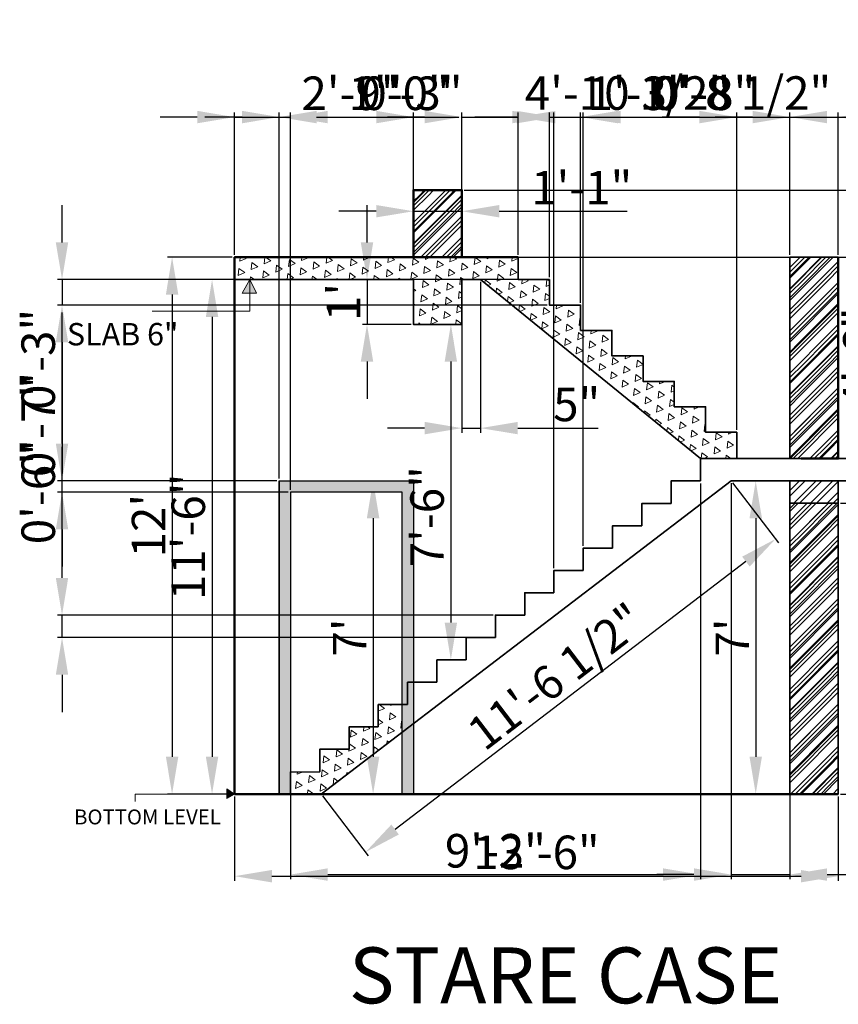
# Model space of a CAD drawing. Units: inches. Extents: x -571 to -216, y 105 to 370.
# Tile 1 of 2: x -571 to -351, y 105 to 370. Entities that reach past the tile are written whole.
import ezdxf

# ---------------------------------------------------------------- set-up
doc = ezdxf.new("R2010")
doc.units = ezdxf.units.IN
for name, color, linetype, lineweight in [('A-ANNO-DIMS', 2, 'Continuous', 18), ('A-ANNO-SYMB', 3, 'Continuous', 18), ('A-ANNO-TEXT', 7, 'Continuous', 18), ('A-DOOR', 4, 'Continuous', 25), ('A-DOOR-PATT', 8, 'Continuous', 13), ('A-FLOR-STRS', 7, 'Continuous', 35), ('A-SECT-PATT', 8, 'Continuous', 18), ('A-WALL', 7, 'Continuous', 50), ('A-WALL-PATT', 8, 'Continuous', 18), ('S-BEAM', 1, 'Continuous', 35)]:
    doc.layers.add(name, color=color, linetype=linetype, lineweight=lineweight)
doc.styles.get("Standard").update_dxf_attribs({"font": 'arial.ttf'})
doc.dimstyles.new('ISO-25', dxfattribs={"dimtxt": 9, "dimasz": 10, "dimexe": 1.25, "dimexo": 0.625, "dimtad": 1, "dimdec": 0, "dimlunit": 3, "dimtxsty": 'Standard', "dimcen": 2.5, "dimadec": 0, "dimazin": 0, "dimtfac": 1, "dimtdec": 0, "dimtmove": 0, "dimatfit": 3, "dimfxl": 1, "dimarcsym": 0})
pattern_1 = [(45, (0, 0), (-2.245064, 2.245064), []), (45, (0, 1.5875), (-2.245064, 2.245064), [])]

# ---------------------------------------------------------------- blocks, each defined once
blk = doc.blocks.new('*D1')
at = {"layer": 'A-ANNO-DIMS', "color": 0, "lineweight": -2, "transparency": 16777216}
for p, q in [((-350.83, 305.84), (-338.04, 305.84)), ((-339.29, 295.84), (-339.29, 261.84)), ((-350.83, 251.84), (-338.04, 251.84))]:
    blk.add_line(p, q, dxfattribs=at)
at = {"layer": 'A-ANNO-DIMS', "color": 0, "transparency": 16777216}
for points in [[(-340.95, 295.84), (-337.62, 295.84), (-339.29, 305.84)], [(-340.95, 261.84), (-337.62, 261.84), (-339.29, 251.84)]]:
    blk.add_solid(points, dxfattribs=at)
at = {"layer": 'Defpoints', "color": 0, "transparency": 16777216}
for p in [(-351.46, 305.84), (-351.46, 251.84), (-339.29, 251.84)]:
    blk.add_point(p, dxfattribs=at)
at = {"layer": 'A-ANNO-DIMS', "color": 0, "transparency": 16777216, "insert": (-344.51, 278.84), "char_height": 9, "attachment_point": 5, "rotation": 90}
blk.add_mtext('4\'-6"', dxfattribs=at)
blk = doc.blocks.new('*D2')
at = {"layer": 'A-ANNO-DIMS', "color": 0, "lineweight": -2, "transparency": 16777216}
for p, q in [((-352.08, 245.84), (-374.87, 245.84)), ((-373.62, 235.84), (-373.62, 171.84)), ((-352.08, 161.84), (-374.87, 161.84))]:
    blk.add_line(p, q, dxfattribs=at)
at = {"layer": 'A-ANNO-DIMS', "color": 0, "transparency": 16777216}
for points in [[(-375.28, 235.84), (-371.95, 235.84), (-373.62, 245.84)], [(-375.28, 171.84), (-371.95, 171.84), (-373.62, 161.84)]]:
    blk.add_solid(points, dxfattribs=at)
at = {"layer": 'Defpoints', "color": 0, "transparency": 16777216}
for p in [(-351.46, 245.84), (-373.62, 161.84), (-351.46, 161.84)]:
    blk.add_point(p, dxfattribs=at)
at = {"layer": 'A-ANNO-DIMS', "color": 0, "transparency": 16777216, "insert": (-378.74, 203.84), "char_height": 9, "attachment_point": 5, "rotation": 90}
blk.add_mtext("7'", dxfattribs=at)
blk = doc.blocks.new('*D3')
at = {"layer": 'A-ANNO-DIMS', "color": 0, "lineweight": -2, "transparency": 16777216}
for p, q in [((-350.83, 239.84), (-327.55, 239.84)), ((-328.8, 229.84), (-328.8, 171.84)), ((-350.83, 161.84), (-327.55, 161.84))]:
    blk.add_line(p, q, dxfattribs=at)
at = {"layer": 'A-ANNO-DIMS', "color": 0, "transparency": 16777216}
for points in [[(-330.47, 229.84), (-327.13, 229.84), (-328.8, 239.84)], [(-330.47, 171.84), (-327.13, 171.84), (-328.8, 161.84)]]:
    blk.add_solid(points, dxfattribs=at)
at = {"layer": 'Defpoints', "color": 0, "transparency": 16777216}
for p in [(-351.46, 239.84), (-351.46, 161.84), (-328.8, 161.84)]:
    blk.add_point(p, dxfattribs=at)
at = {"layer": 'A-ANNO-DIMS', "color": 0, "transparency": 16777216, "insert": (-334.02, 200.84), "char_height": 9, "attachment_point": 5, "rotation": 90}
blk.add_mtext('6\'-6"', dxfattribs=at)
blk = doc.blocks.new('*D5')
at = {"layer": 'A-ANNO-DIMS', "color": 0, "lineweight": -2, "transparency": 16777216}
for p, q in [((-513.46, 161.21), (-513.46, 138.56)), ((-351.46, 161.21), (-351.46, 138.56)), ((-503.46, 139.81), (-361.46, 139.81))]:
    blk.add_line(p, q, dxfattribs=at)
at = {"layer": 'A-ANNO-DIMS', "color": 0, "transparency": 16777216}
for points in [[(-503.46, 141.47), (-503.46, 138.14), (-513.46, 139.81)], [(-361.46, 141.47), (-361.46, 138.14), (-351.46, 139.81)]]:
    blk.add_solid(points, dxfattribs=at)
at = {"layer": 'Defpoints', "color": 0, "transparency": 16777216}
for p in [(-513.46, 161.84), (-351.46, 161.84), (-351.46, 139.81)]:
    blk.add_point(p, dxfattribs=at)
at = {"layer": 'A-ANNO-DIMS', "color": 0, "transparency": 16777216, "insert": (-432.46, 145.03), "char_height": 9, "attachment_point": 5}
blk.add_mtext('13\'-6"', dxfattribs=at)
blk = doc.blocks.new('*D6')
at = {"layer": 'A-ANNO-DIMS', "color": 0, "lineweight": -2, "transparency": 16777216}
for p, q in [((-482.83, 245.84), (-475.04, 245.84)), ((-476.29, 235.84), (-476.29, 171.84)), ((-482.83, 161.84), (-475.04, 161.84))]:
    blk.add_line(p, q, dxfattribs=at)
at = {"layer": 'A-ANNO-DIMS', "color": 0, "transparency": 16777216}
for points in [[(-477.96, 235.84), (-474.62, 235.84), (-476.29, 245.84)], [(-477.96, 171.84), (-474.62, 171.84), (-476.29, 161.84)]]:
    blk.add_solid(points, dxfattribs=at)
at = {"layer": 'Defpoints', "color": 0, "transparency": 16777216}
for p in [(-483.46, 245.84), (-483.46, 161.84), (-476.29, 161.84)]:
    blk.add_point(p, dxfattribs=at)
at = {"layer": 'A-ANNO-DIMS', "color": 0, "transparency": 16777216, "insert": (-481.42, 203.84), "char_height": 9, "attachment_point": 5, "rotation": 90}
blk.add_mtext("7'", dxfattribs=at)
blk = doc.blocks.new('*D7')
at = {"layer": 'A-ANNO-DIMS', "color": 0, "lineweight": -2, "transparency": 16777216}
for p, q in [((-458.33, 287.84), (-454.17, 287.84)), ((-455.42, 277.84), (-455.42, 207.83)), ((-458.55, 197.83), (-454.17, 197.83))]:
    blk.add_line(p, q, dxfattribs=at)
at = {"layer": 'A-ANNO-DIMS', "color": 0, "transparency": 16777216}
for points in [[(-457.09, 277.84), (-453.76, 277.84), (-455.42, 287.84)], [(-457.09, 207.83), (-453.76, 207.83), (-455.42, 197.83)]]:
    blk.add_solid(points, dxfattribs=at)
at = {"layer": 'Defpoints', "color": 0, "transparency": 16777216}
for p in [(-458.96, 287.84), (-459.17, 197.83), (-455.42, 197.83)]:
    blk.add_point(p, dxfattribs=at)
at = {"layer": 'A-ANNO-DIMS', "color": 0, "transparency": 16777216, "insert": (-460.65, 236.23), "char_height": 9, "attachment_point": 5, "rotation": 90}
blk.add_mtext('7\'-6"', dxfattribs=at)
blk = doc.blocks.new('*D8')
at = {"layer": 'A-ANNO-DIMS', "color": 0, "lineweight": -2, "transparency": 16777216}
for p, q in [((-514.08, 305.84), (-531.48, 305.84)), ((-530.23, 295.84), (-530.23, 171.84)), ((-514.08, 161.84), (-531.48, 161.84))]:
    blk.add_line(p, q, dxfattribs=at)
at = {"layer": 'A-ANNO-DIMS', "color": 0, "transparency": 16777216}
for points in [[(-531.89, 295.84), (-528.56, 295.84), (-530.23, 305.84)], [(-531.89, 171.84), (-528.56, 171.84), (-530.23, 161.84)]]:
    blk.add_solid(points, dxfattribs=at)
at = {"layer": 'Defpoints', "color": 0, "transparency": 16777216}
for p in [(-513.46, 305.84), (-530.23, 161.84), (-513.46, 161.84)]:
    blk.add_point(p, dxfattribs=at)
at = {"layer": 'A-ANNO-DIMS', "color": 0, "transparency": 16777216, "insert": (-535.37, 233.84), "char_height": 9, "attachment_point": 5, "rotation": 90}
blk.add_mtext("12'", dxfattribs=at)
blk = doc.blocks.new('*D9')
at = {"layer": 'A-ANNO-DIMS', "color": 0, "lineweight": -2, "transparency": 16777216}
for p, q in [((-514.08, 299.84), (-520.75, 299.84)), ((-519.5, 289.84), (-519.5, 171.84)), ((-514.08, 161.84), (-520.75, 161.84))]:
    blk.add_line(p, q, dxfattribs=at)
at = {"layer": 'A-ANNO-DIMS', "color": 0, "transparency": 16777216}
for points in [[(-521.17, 289.84), (-517.84, 289.84), (-519.5, 299.84)], [(-521.17, 171.84), (-517.84, 171.84), (-519.5, 161.84)]]:
    blk.add_solid(points, dxfattribs=at)
at = {"layer": 'Defpoints', "color": 0, "transparency": 16777216}
for p in [(-513.46, 299.84), (-519.5, 161.84), (-513.46, 161.84)]:
    blk.add_point(p, dxfattribs=at)
at = {"layer": 'A-ANNO-DIMS', "color": 0, "transparency": 16777216, "insert": (-524.73, 230.84), "char_height": 9, "attachment_point": 5, "rotation": 90}
blk.add_mtext('11\'-6"', dxfattribs=at)
blk = doc.blocks.new('*D10')
at = {"layer": 'A-ANNO-DIMS', "color": 0, "lineweight": -2, "transparency": 16777216}
for p, q in [((-477.92, 309.84), (-477.92, 319.84)), ((-466.08, 299.84), (-479.17, 299.84)), ((-477.92, 299.84), (-477.92, 287.84)), ((-466.08, 287.84), (-479.17, 287.84)), ((-477.92, 277.84), (-477.92, 267.84))]:
    blk.add_line(p, q, dxfattribs=at)
at = {"layer": 'A-ANNO-DIMS', "color": 0, "transparency": 16777216}
for points in [[(-479.59, 309.84), (-476.26, 309.84), (-477.92, 299.84)], [(-479.59, 277.84), (-476.26, 277.84), (-477.92, 287.84)]]:
    blk.add_solid(points, dxfattribs=at)
at = {"layer": 'Defpoints', "color": 0, "transparency": 16777216}
for p in [(-465.46, 299.84), (-477.92, 287.84), (-465.46, 287.84)]:
    blk.add_point(p, dxfattribs=at)
at = {"layer": 'A-ANNO-DIMS', "color": 0, "transparency": 16777216, "insert": (-483.07, 293.84), "char_height": 9, "attachment_point": 5, "rotation": 90}
blk.add_mtext("1'", dxfattribs=at)
blk = doc.blocks.new('*D11')
at = {"layer": 'A-ANNO-DIMS', "color": 0, "lineweight": -2, "transparency": 16777216}
for p, q in [((-465.46, 323.21), (-465.46, 316.93)), ((-452.46, 323.21), (-452.46, 316.93)), ((-475.46, 318.18), (-485.46, 318.18)), ((-465.46, 318.18), (-452.46, 318.18)), ((-442.46, 318.18), (-408.13, 318.18))]:
    blk.add_line(p, q, dxfattribs=at)
at = {"layer": 'A-ANNO-DIMS', "color": 0, "transparency": 16777216}
for points in [[(-475.46, 319.85), (-475.46, 316.52), (-465.46, 318.18)], [(-442.46, 319.85), (-442.46, 316.52), (-452.46, 318.18)]]:
    blk.add_solid(points, dxfattribs=at)
at = {"layer": 'Defpoints', "color": 0, "transparency": 16777216}
for p in [(-465.46, 323.84), (-452.46, 323.84), (-452.46, 318.18)]:
    blk.add_point(p, dxfattribs=at)
at = {"layer": 'A-ANNO-DIMS', "color": 0, "transparency": 16777216, "insert": (-420.3, 323.33), "char_height": 9, "attachment_point": 5}
blk.add_mtext('1\'-1"', dxfattribs=at)
blk = doc.blocks.new('*D12')
at = {"layer": 'A-ANNO-DIMS', "color": 0, "lineweight": -2, "transparency": 16777216}
for p, q in [((-452.46, 299.21), (-452.46, 258.75)), ((-447.46, 299.21), (-447.46, 258.75)), ((-462.46, 260), (-472.46, 260)), ((-452.46, 260), (-447.46, 260)), ((-437.46, 260), (-415.87, 260))]:
    blk.add_line(p, q, dxfattribs=at)
at = {"layer": 'A-ANNO-DIMS', "color": 0, "transparency": 16777216}
for points in [[(-462.46, 261.67), (-462.46, 258.34), (-452.46, 260)], [(-437.46, 261.67), (-437.46, 258.34), (-447.46, 260)]]:
    blk.add_solid(points, dxfattribs=at)
at = {"layer": 'Defpoints', "color": 0, "transparency": 16777216}
for p in [(-452.46, 299.84), (-447.46, 299.84), (-447.46, 260)]:
    blk.add_point(p, dxfattribs=at)
at = {"layer": 'A-ANNO-DIMS', "color": 0, "transparency": 16777216, "insert": (-421.66, 265.2), "char_height": 9, "attachment_point": 5}
blk.add_mtext('5"', dxfattribs=at)
blk = doc.blocks.new('*D13')
at = {"layer": 'A-ANNO-DIMS', "color": 0, "lineweight": -2, "transparency": 16777216}
for p, q in [((-523.46, 343.44), (-533.46, 343.44)), ((-513.46, 306.46), (-513.46, 344.69)), ((-513.46, 343.44), (-501.46, 343.44)), ((-501.46, 246.46), (-501.46, 344.69)), ((-491.46, 343.44), (-457.13, 343.44))]:
    blk.add_line(p, q, dxfattribs=at)
at = {"layer": 'A-ANNO-DIMS', "color": 0, "transparency": 16777216}
for points in [[(-523.46, 345.11), (-523.46, 341.77), (-513.46, 343.44)], [(-491.46, 345.11), (-491.46, 341.77), (-501.46, 343.44)]]:
    blk.add_solid(points, dxfattribs=at)
at = {"layer": 'Defpoints', "color": 0, "transparency": 16777216}
for p in [(-501.46, 343.44), (-513.46, 305.84), (-501.46, 245.84)]:
    blk.add_point(p, dxfattribs=at)
at = {"layer": 'A-ANNO-DIMS', "color": 0, "transparency": 16777216, "insert": (-469.3, 348.66), "char_height": 9, "attachment_point": 5}
blk.add_mtext('1\'-0"', dxfattribs=at)
blk = doc.blocks.new('*D14')
at = {"layer": 'A-ANNO-DIMS', "color": 0, "lineweight": -2, "transparency": 16777216}
for p, q in [((-511.46, 343.44), (-521.46, 343.44)), ((-501.46, 246.46), (-501.46, 344.69)), ((-501.46, 343.44), (-498.46, 343.44)), ((-498.46, 243.46), (-498.46, 344.69)), ((-488.46, 343.44), (-453.29, 343.44))]:
    blk.add_line(p, q, dxfattribs=at)
at = {"layer": 'A-ANNO-DIMS', "color": 0, "transparency": 16777216}
for points in [[(-511.46, 345.11), (-511.46, 341.77), (-501.46, 343.44)], [(-488.46, 345.11), (-488.46, 341.77), (-498.46, 343.44)]]:
    blk.add_solid(points, dxfattribs=at)
at = {"layer": 'Defpoints', "color": 0, "transparency": 16777216}
for p in [(-498.46, 343.44), (-501.46, 245.84), (-498.46, 242.84)]:
    blk.add_point(p, dxfattribs=at)
at = {"layer": 'A-ANNO-DIMS', "color": 0, "transparency": 16777216, "insert": (-465.87, 348.66), "char_height": 9, "attachment_point": 5}
blk.add_mtext('0\'-3"', dxfattribs=at)
blk = doc.blocks.new('*D15')
at = {"layer": 'A-ANNO-DIMS', "color": 0, "lineweight": -2, "transparency": 16777216}
for p, q in [((-498.46, 243.46), (-498.46, 344.69)), ((-488.46, 343.44), (-475.46, 343.44)), ((-465.46, 306.46), (-465.46, 344.69))]:
    blk.add_line(p, q, dxfattribs=at)
at = {"layer": 'A-ANNO-DIMS', "color": 0, "transparency": 16777216}
for points in [[(-488.46, 345.11), (-488.46, 341.77), (-498.46, 343.44)], [(-475.46, 345.11), (-475.46, 341.77), (-465.46, 343.44)]]:
    blk.add_solid(points, dxfattribs=at)
at = {"layer": 'Defpoints', "color": 0, "transparency": 16777216}
for p in [(-465.46, 343.44), (-465.46, 305.84), (-498.46, 242.84)]:
    blk.add_point(p, dxfattribs=at)
at = {"layer": 'A-ANNO-DIMS', "color": 0, "transparency": 16777216, "insert": (-481.96, 348.66), "char_height": 9, "attachment_point": 5}
blk.add_mtext('2\'-9"', dxfattribs=at)
blk = doc.blocks.new('*D16')
at = {"layer": 'A-ANNO-DIMS', "color": 0, "lineweight": -2, "transparency": 16777216}
for p, q in [((-462.46, 343.44), (-472.46, 343.44)), ((-452.46, 306.46), (-452.46, 344.69)), ((-452.46, 343.44), (-437.35, 343.44)), ((-437.35, 306.46), (-437.35, 344.69)), ((-427.35, 343.44), (-393.02, 343.44))]:
    blk.add_line(p, q, dxfattribs=at)
at = {"layer": 'A-ANNO-DIMS', "color": 0, "transparency": 16777216}
for points in [[(-462.46, 345.11), (-462.46, 341.77), (-452.46, 343.44)], [(-427.35, 345.11), (-427.35, 341.77), (-437.35, 343.44)]]:
    blk.add_solid(points, dxfattribs=at)
at = {"layer": 'Defpoints', "color": 0, "transparency": 16777216}
for p in [(-437.35, 343.44), (-452.46, 305.84), (-437.35, 305.84)]:
    blk.add_point(p, dxfattribs=at)
at = {"layer": 'A-ANNO-DIMS', "color": 0, "transparency": 16777216, "insert": (-405.19, 348.66), "char_height": 9, "attachment_point": 5}
blk.add_mtext('1\'-3"', dxfattribs=at)
blk = doc.blocks.new('*D17')
at = {"layer": 'A-ANNO-DIMS', "color": 0, "lineweight": -2, "transparency": 16777216}
for p, q in [((-437.35, 306.46), (-437.35, 344.69)), ((-427.35, 343.44), (-388.71, 343.44)), ((-378.71, 259.52), (-378.71, 344.69))]:
    blk.add_line(p, q, dxfattribs=at)
at = {"layer": 'A-ANNO-DIMS', "color": 0, "transparency": 16777216}
for points in [[(-427.35, 345.11), (-427.35, 341.77), (-437.35, 343.44)], [(-388.71, 345.11), (-388.71, 341.77), (-378.71, 343.44)]]:
    blk.add_solid(points, dxfattribs=at)
at = {"layer": 'Defpoints', "color": 0, "transparency": 16777216}
for p in [(-378.71, 343.44), (-437.35, 305.84), (-378.71, 258.89)]:
    blk.add_point(p, dxfattribs=at)
at = {"layer": 'A-ANNO-DIMS', "color": 0, "transparency": 16777216, "insert": (-408.03, 348.72), "char_height": 9, "attachment_point": 5}
blk.add_mtext('4\'-10 1/2"', dxfattribs=at)
blk = doc.blocks.new('*D18')
at = {"layer": 'A-ANNO-DIMS', "color": 0, "lineweight": -2, "transparency": 16777216}
for p, q in [((-388.71, 343.44), (-398.71, 343.44)), ((-378.71, 259.52), (-378.71, 344.69)), ((-378.71, 343.44), (-364.46, 343.44)), ((-364.46, 306.46), (-364.46, 344.69)), ((-354.46, 343.44), (-299.16, 343.44))]:
    blk.add_line(p, q, dxfattribs=at)
at = {"layer": 'A-ANNO-DIMS', "color": 0, "transparency": 16777216}
for points in [[(-388.71, 345.11), (-388.71, 341.77), (-378.71, 343.44)], [(-354.46, 345.11), (-354.46, 341.77), (-364.46, 343.44)]]:
    blk.add_solid(points, dxfattribs=at)
at = {"layer": 'Defpoints', "color": 0, "transparency": 16777216}
for p in [(-364.46, 343.44), (-364.46, 305.84), (-378.71, 258.89)]:
    blk.add_point(p, dxfattribs=at)
at = {"layer": 'A-ANNO-DIMS', "color": 0, "transparency": 16777216, "insert": (-321.81, 348.72), "char_height": 9, "attachment_point": 5}
blk.add_mtext('1\'-2 1/2"', dxfattribs=at)
blk = doc.blocks.new('*D19')
at = {"layer": 'A-ANNO-DIMS', "color": 0, "lineweight": -2, "transparency": 16777216}
for p, q in [((-374.46, 343.44), (-384.46, 343.44)), ((-364.46, 306.46), (-364.46, 344.69)), ((-364.46, 343.44), (-351.46, 343.44)), ((-351.46, 306.46), (-351.46, 344.69)), ((-341.46, 343.44), (-307.13, 343.44))]:
    blk.add_line(p, q, dxfattribs=at)
at = {"layer": 'A-ANNO-DIMS', "color": 0, "transparency": 16777216}
for points in [[(-374.46, 345.11), (-374.46, 341.77), (-364.46, 343.44)], [(-341.46, 345.11), (-341.46, 341.77), (-351.46, 343.44)]]:
    blk.add_solid(points, dxfattribs=at)
at = {"layer": 'Defpoints', "color": 0, "transparency": 16777216}
for p in [(-351.46, 343.44), (-364.46, 305.84), (-351.46, 305.84)]:
    blk.add_point(p, dxfattribs=at)
at = {"layer": 'A-ANNO-DIMS', "color": 0, "transparency": 16777216, "insert": (-319.3, 348.58), "char_height": 9, "attachment_point": 5}
blk.add_mtext('1\'-1"', dxfattribs=at)
blk = doc.blocks.new('*D21')
at = {"layer": 'A-ANNO-DIMS', "color": 0, "lineweight": -2, "transparency": 16777216}
for p, q in [((-265.01, 333.84), (-265.01, 368.17)), ((-451.83, 323.84), (-263.76, 323.84)), ((-265.01, 305.84), (-265.01, 323.84)), ((-451.83, 305.84), (-263.76, 305.84)), ((-265.01, 295.84), (-265.01, 285.84))]:
    blk.add_line(p, q, dxfattribs=at)
at = {"layer": 'A-ANNO-DIMS', "color": 0, "transparency": 16777216}
for points in [[(-266.68, 333.84), (-263.35, 333.84), (-265.01, 323.84)], [(-266.68, 295.84), (-263.35, 295.84), (-265.01, 305.84)]]:
    blk.add_solid(points, dxfattribs=at)
at = {"layer": 'Defpoints', "color": 0, "transparency": 16777216}
for p in [(-452.46, 323.84), (-265.01, 323.84), (-452.46, 305.84)]:
    blk.add_point(p, dxfattribs=at)
at = {"layer": 'A-ANNO-DIMS', "color": 0, "transparency": 16777216, "insert": (-270.23, 356), "char_height": 9, "attachment_point": 5, "rotation": 90}
blk.add_mtext('1\'-6"', dxfattribs=at)
blk = doc.blocks.new('*D22')
at = {"layer": 'A-ANNO-DIMS', "color": 0, "lineweight": -2, "transparency": 16777216}
for p, q in [((-438.97, 343.44), (-448.97, 343.44)), ((-428.97, 300.47), (-428.97, 344.69)), ((-428.97, 343.44), (-420.6, 343.44)), ((-420.6, 293.64), (-420.6, 344.69)), ((-410.6, 343.44), (-354.45, 343.44))]:
    blk.add_line(p, q, dxfattribs=at)
at = {"layer": 'A-ANNO-DIMS', "color": 0, "transparency": 16777216}
for points in [[(-438.97, 345.11), (-438.97, 341.77), (-428.97, 343.44)], [(-410.6, 345.11), (-410.6, 341.77), (-420.6, 343.44)]]:
    blk.add_solid(points, dxfattribs=at)
at = {"layer": 'Defpoints', "color": 0, "transparency": 16777216}
for p in [(-420.6, 343.44), (-428.97, 299.84), (-420.6, 293.02)]:
    blk.add_point(p, dxfattribs=at)
at = {"layer": 'A-ANNO-DIMS', "color": 0, "transparency": 16777216, "insert": (-377.52, 348.72), "char_height": 9, "attachment_point": 5}
blk.add_mtext('0\'-8 1/2"', dxfattribs=at)
blk = doc.blocks.new('*D23')
at = {"layer": 'A-ANNO-DIMS', "color": 0, "lineweight": -2, "transparency": 16777216}
for p, q in [((-559.76, 309.84), (-559.76, 319.84)), ((-429.6, 299.84), (-561.01, 299.84)), ((-559.76, 299.84), (-559.76, 293.02)), ((-429.6, 293.02), (-561.01, 293.02)), ((-559.76, 283.02), (-559.76, 247.84))]:
    blk.add_line(p, q, dxfattribs=at)
at = {"layer": 'A-ANNO-DIMS', "color": 0, "transparency": 16777216}
for points in [[(-561.43, 309.84), (-558.1, 309.84), (-559.76, 299.84)], [(-561.43, 283.02), (-558.1, 283.02), (-559.76, 293.02)]]:
    blk.add_solid(points, dxfattribs=at)
at = {"layer": 'Defpoints', "color": 0, "transparency": 16777216}
for p in [(-428.97, 299.84), (-559.76, 293.02), (-428.97, 293.02)]:
    blk.add_point(p, dxfattribs=at)
at = {"layer": 'A-ANNO-DIMS', "color": 0, "transparency": 16777216, "insert": (-564.98, 260.43), "char_height": 9, "attachment_point": 5, "rotation": 90}
blk.add_mtext('0\'-7"', dxfattribs=at)
blk = doc.blocks.new('*D26')
at = {"layer": 'A-ANNO-DIMS', "color": 0, "lineweight": -2, "transparency": 16777216}
for p, q in [((-380.19, 245.21), (-380.19, 138.99)), ((-364.46, 245.21), (-364.46, 138.99)), ((-390.19, 140.24), (-400.19, 140.24)), ((-380.19, 140.24), (-364.46, 140.24)), ((-354.46, 140.24), (-299.16, 140.24))]:
    blk.add_line(p, q, dxfattribs=at)
at = {"layer": 'A-ANNO-DIMS', "color": 0, "transparency": 16777216}
for points in [[(-390.19, 141.91), (-390.19, 138.57), (-380.19, 140.24)], [(-354.46, 141.91), (-354.46, 138.57), (-364.46, 140.24)]]:
    blk.add_solid(points, dxfattribs=at)
at = {"layer": 'Defpoints', "color": 0, "transparency": 16777216}
for p in [(-380.19, 245.84), (-364.46, 245.84), (-364.46, 140.24)]:
    blk.add_point(p, dxfattribs=at)
at = {"layer": 'A-ANNO-DIMS', "color": 0, "transparency": 16777216, "insert": (-321.81, 145.52), "char_height": 9, "attachment_point": 5}
blk.add_mtext('1\'-3 1/2"', dxfattribs=at)
blk = doc.blocks.new('*D27')
at = {"layer": 'A-ANNO-DIMS', "color": 0, "lineweight": -2, "transparency": 16777216}
for p, q in [((-388.46, 245.19), (-388.46, 138.99)), ((-498.46, 167.21), (-498.46, 138.99)), ((-488.46, 140.24), (-398.46, 140.24))]:
    blk.add_line(p, q, dxfattribs=at)
at = {"layer": 'A-ANNO-DIMS', "color": 0, "transparency": 16777216}
for points in [[(-488.46, 141.91), (-488.46, 138.57), (-498.46, 140.24)], [(-398.46, 141.91), (-398.46, 138.57), (-388.46, 140.24)]]:
    blk.add_solid(points, dxfattribs=at)
at = {"layer": 'Defpoints', "color": 0, "transparency": 16777216}
for p in [(-388.46, 245.82), (-498.46, 167.84), (-388.46, 140.24)]:
    blk.add_point(p, dxfattribs=at)
at = {"layer": 'A-ANNO-DIMS', "color": 0, "transparency": 16777216, "insert": (-443.46, 145.46), "char_height": 9, "attachment_point": 5}
blk.add_mtext('9\'-2"', dxfattribs=at)
blk = doc.blocks.new('*D28')
at = {"layer": 'A-ANNO-DIMS', "color": 0, "lineweight": -2, "transparency": 16777216}
for p, q in [((-379.81, 245.34), (-367.54, 229.27)), ((-376.25, 224.19), (-470.38, 152.33)), ((-489.84, 161.34), (-477.57, 145.27))]:
    blk.add_line(p, q, dxfattribs=at)
at = {"layer": 'A-ANNO-DIMS', "color": 0, "transparency": 16777216}
for points in [[(-377.26, 225.52), (-375.24, 222.87), (-368.3, 230.26)], [(-471.39, 153.65), (-469.37, 151), (-478.33, 146.26)]]:
    blk.add_solid(points, dxfattribs=at)
at = {"layer": 'Defpoints', "color": 0, "transparency": 16777216}
for p in [(-380.19, 245.84), (-490.22, 161.84), (-478.33, 146.26)]:
    blk.add_point(p, dxfattribs=at)
at = {"layer": 'A-ANNO-DIMS', "color": 0, "transparency": 16777216, "insert": (-426.52, 192.46), "char_height": 9, "attachment_point": 5, "rotation": 37.3595}
blk.add_mtext('11\'-6 1/2"', dxfattribs=at)
blk = doc.blocks.new('*D29')
at = {"layer": 'A-ANNO-DIMS', "color": 0, "lineweight": -2, "transparency": 16777216}
for p, q in [((-437.75, 343.44), (-447.75, 343.44)), ((-427.75, 222.45), (-427.75, 344.69)), ((-427.75, 343.44), (-419.89, 343.44)), ((-419.89, 228.45), (-419.89, 344.69)), ((-409.89, 343.44), (-374.72, 343.44))]:
    blk.add_line(p, q, dxfattribs=at)
at = {"layer": 'A-ANNO-DIMS', "color": 0, "transparency": 16777216}
for points in [[(-437.75, 345.11), (-437.75, 341.77), (-427.75, 343.44)], [(-409.89, 345.11), (-409.89, 341.77), (-419.89, 343.44)]]:
    blk.add_solid(points, dxfattribs=at)
at = {"layer": 'Defpoints', "color": 0, "transparency": 16777216}
for p in [(-419.89, 343.44), (-419.89, 227.82), (-427.75, 221.82)]:
    blk.add_point(p, dxfattribs=at)
at = {"layer": 'A-ANNO-DIMS', "color": 0, "transparency": 16777216, "insert": (-387.3, 348.66), "char_height": 9, "attachment_point": 5}
blk.add_mtext('0\'-8"', dxfattribs=at)
blk = doc.blocks.new('*D30')
at = {"layer": 'A-ANNO-DIMS', "color": 0, "lineweight": -2, "transparency": 16777216}
for p, q in [((-559.76, 219.83), (-559.76, 255)), ((-444.09, 209.83), (-561.01, 209.83)), ((-559.76, 203.83), (-559.76, 209.83)), ((-444.09, 203.83), (-561.01, 203.83)), ((-559.76, 193.83), (-559.76, 183.83))]:
    blk.add_line(p, q, dxfattribs=at)
at = {"layer": 'A-ANNO-DIMS', "color": 0, "transparency": 16777216}
for points in [[(-561.43, 219.83), (-558.1, 219.83), (-559.76, 209.83)], [(-561.43, 193.83), (-558.1, 193.83), (-559.76, 203.83)]]:
    blk.add_solid(points, dxfattribs=at)
at = {"layer": 'Defpoints', "color": 0, "transparency": 16777216}
for p in [(-559.76, 209.83), (-443.46, 209.83), (-443.46, 203.83)]:
    blk.add_point(p, dxfattribs=at)
at = {"layer": 'A-ANNO-DIMS', "color": 0, "transparency": 16777216, "insert": (-564.98, 242.41), "char_height": 9, "attachment_point": 5, "rotation": 90}
blk.add_mtext('0\'-6"', dxfattribs=at)
blk = doc.blocks.new('*D31')
at = {"layer": 'A-ANNO-DIMS', "color": 0, "lineweight": -2, "transparency": 16777216}
for p, q in [((-559.76, 255.84), (-559.76, 291.01)), ((-502.08, 245.84), (-561.01, 245.84)), ((-559.76, 242.84), (-559.76, 245.84)), ((-499.08, 242.84), (-561.01, 242.84)), ((-559.76, 232.84), (-559.76, 222.84))]:
    blk.add_line(p, q, dxfattribs=at)
at = {"layer": 'A-ANNO-DIMS', "color": 0, "transparency": 16777216}
for points in [[(-561.43, 255.84), (-558.1, 255.84), (-559.76, 245.84)], [(-561.43, 232.84), (-558.1, 232.84), (-559.76, 242.84)]]:
    blk.add_solid(points, dxfattribs=at)
at = {"layer": 'Defpoints', "color": 0, "transparency": 16777216}
for p in [(-559.76, 245.84), (-501.46, 245.84), (-498.46, 242.84)]:
    blk.add_point(p, dxfattribs=at)
at = {"layer": 'A-ANNO-DIMS', "color": 0, "transparency": 16777216, "insert": (-564.99, 278.43), "char_height": 9, "attachment_point": 5, "rotation": 90}
blk.add_mtext('0\'-3"', dxfattribs=at)

msp = doc.modelspace()

# ---------------------------------------------------------------- hatches: boundary and pattern name
at = {"layer": 'A-ANNO-SYMB'}
h = msp.add_hatch(color=256, dxfattribs=at)
h.dxf.hatch_style = 1
h.paths.add_polyline_path([(-509.37, 296.17), (-509.37, 299.84), (-511.42, 296.17)])
h = msp.add_hatch(color=256, dxfattribs=at)
h.dxf.hatch_style = 1
h.paths.add_polyline_path([(-509.37, 296.17), (-507.58, 296.17), (-509.37, 299.84)])
h = msp.add_hatch(color=256, dxfattribs=at)
h.dxf.hatch_style = 1
h.paths.add_polyline_path([(-515.51, 163.25), (-515.51, 161.84), (-513.46, 161.84)])
h = msp.add_hatch(color=256, dxfattribs=at)
h.dxf.hatch_style = 1
h.paths.add_polyline_path([(-515.51, 161.84), (-515.51, 160.69), (-513.46, 161.84)])
at = {"layer": 'A-DOOR-PATT'}
h = msp.add_hatch(color=256, dxfattribs=at)
h.dxf.hatch_style = 1
h.paths.add_polyline_path([(-498.46, 242.84), (-468.46, 242.84), (-468.46, 185.83), (-467.03, 185.83), (-467.03, 191.83), (-465.46, 191.83), (-465.46, 245.84), (-501.46, 245.84), (-501.46, 161.84), (-498.46, 161.84)])
h.paths.add_polyline_path([(-451.29, 221.46), (-451.29, 250.99), (-469.84, 250.99), (-469.84, 221.46)], flags=9)
h = msp.add_hatch(color=256, dxfattribs=at)
h.dxf.hatch_style = 1
h.paths.add_polyline_path([(-501.46, 245.84), (-501.46, 161.84), (-498.46, 161.84), (-498.46, 242.84), (-468.46, 242.84), (-468.46, 185.83), (-467.03, 185.83), (-467.03, 191.83), (-465.46, 191.83), (-465.46, 245.84)])
h.paths.add_polyline_path([(-451.29, 221.46), (-451.29, 250.99), (-469.84, 250.99), (-469.84, 221.46)], flags=9)
h = msp.add_hatch(color=256, dxfattribs=at)
h.dxf.hatch_style = 1
h.paths.add_polyline_path([(-465.46, 245.84), (-501.46, 245.84), (-501.46, 161.84), (-498.46, 161.84), (-498.46, 242.84), (-468.46, 242.84), (-468.46, 185.83), (-467.03, 185.83), (-467.03, 191.83), (-465.46, 191.83)])
h.paths.add_polyline_path([(-451.29, 221.46), (-451.29, 250.99), (-469.84, 250.99), (-469.84, 221.46)], flags=9)
h = msp.add_hatch(color=256, dxfattribs=at)
h.dxf.hatch_style = 1
h.paths.add_polyline_path([(-465.46, 245.84), (-501.46, 245.84), (-501.46, 161.84), (-498.46, 161.84), (-498.46, 242.84), (-468.46, 242.84), (-468.46, 178.45), (-465.46, 180.74)])
h = msp.add_hatch(color=256, dxfattribs=at)
h.dxf.hatch_style = 1
h.paths.add_polyline_path([(-468.46, 161.84), (-465.46, 161.84), (-465.46, 180.74), (-468.46, 178.45)])
at = {"layer": 'A-SECT-PATT'}
h = msp.add_hatch(dxfattribs=at)
h.set_pattern_fill('TRIANG', color=256, scale=0.4, angle=204)
h.paths.add_polyline_path([(-437.35, 305.84), (-513.46, 305.84), (-513.46, 299.84), (-465.46, 299.84), (-465.46, 287.84), (-452.46, 287.84), (-452.46, 299.84), (-447.46, 299.84), (-388.49, 251.84), (-378.71, 251.84), (-378.71, 258.89), (-387.09, 258.89), (-387.09, 265.72), (-395.47, 265.72), (-395.47, 272.54), (-403.84, 272.54), (-403.84, 279.37), (-412.22, 279.37), (-412.22, 286.19), (-420.6, 286.19), (-420.6, 293.02), (-428.97, 293.02), (-428.97, 299.84), (-437.35, 299.84)])
h = msp.add_hatch(dxfattribs=at)
h.set_pattern_fill('STEEL', color=256)
h.set_pattern_definition(pattern_1)
h.paths.add_polyline_path([(-364.46, 245.84), (-364.46, 239.84), (-351.46, 239.84), (-351.46, 245.84)])
h = msp.add_hatch(dxfattribs=at)
h.set_pattern_fill('STEEL', color=256)
h.set_pattern_definition(pattern_1)
h.paths.add_polyline_path([(-364.46, 245.84), (-364.46, 239.84), (-351.46, 239.84), (-351.46, 245.84)])
h = msp.add_hatch(dxfattribs=at)
h.set_pattern_fill('TRIANG', color=256, scale=0.4, angle=204)
h.paths.add_polyline_path([(-468.46, 178.45), (-468.46, 185.83), (-474.89, 185.83), (-474.89, 179.84), (-482.75, 179.84), (-482.75, 173.84), (-490.6, 173.84), (-490.6, 167.84), (-498.46, 167.84), (-498.46, 161.84), (-490.22, 161.84)])
at = {"layer": 'A-WALL-PATT'}
h = msp.add_hatch(dxfattribs=at)
h.set_pattern_fill('GOST_GROUND', color=256)
h.paths.add_polyline_path([(-351.46, 305.84), (-364.46, 305.84), (-364.46, 251.84), (-351.46, 251.84)])
h.paths.add_polyline_path([(-351.46, 239.84), (-364.46, 239.84), (-364.46, 161.84), (-351.46, 161.84)])
h.paths.add_polyline_path([(-306.8, 275.84), (-312.8, 275.84), (-312.8, 251.84), (-306.8, 251.84)])
h.paths.add_polyline_path([(-452.46, 323.84), (-465.46, 323.84), (-465.46, 305.84), (-452.46, 305.84)])
h = msp.add_hatch(dxfattribs=at)
h.set_pattern_fill('GOST_GROUND', color=256, scale=0.4)
h.paths.add_polyline_path([(-351.46, 305.84), (-364.46, 305.84), (-364.46, 251.84), (-351.46, 251.84)])
h.paths.add_polyline_path([(-351.46, 239.84), (-364.46, 239.84), (-364.46, 161.84), (-351.46, 161.84)])
h.paths.add_polyline_path([(-452.46, 323.84), (-465.46, 323.84), (-465.46, 305.84), (-452.46, 305.84)])
h.paths.add_polyline_path([(-306.8, 275.84), (-312.8, 275.84), (-312.8, 251.84), (-306.8, 251.84)])

# ---------------------------------------------------------------- linework, layer by layer
at = {"layer": 'A-ANNO-SYMB'}
for p, q in [((-509.37, 299.84), (-511.42, 296.17)), ((-509.37, 299.84), (-509.37, 291.4)), ((-509.37, 299.84), (-509.37, 299.84)), ((-507.58, 296.17), (-509.37, 299.84)), ((-511.42, 296.17), (-507.58, 296.17)), ((-509.37, 291.4), (-535.58, 291.4)), ((-513.46, 161.84), (-540.16, 161.84)), ((-540.16, 161.84), (-540.16, 159.84)), ((-513.46, 161.84), (-515.97, 161.84)), ((-513.46, 161.84), (-515.51, 163.25)), ((-515.51, 163.25), (-515.51, 160.69)), ((-515.51, 160.69), (-513.46, 161.84))]:
    msp.add_line(p, q, dxfattribs=at)
at = {"layer": 'A-DOOR'}
for points in [[(-501.46, 245.84), (-501.46, 161.84), (-501.46, 245.84), (-465.46, 245.84), (-465.46, 161.84)], [(-468.46, 161.84), (-468.46, 242.84), (-498.46, 242.84), (-498.46, 161.84), (-498.46, 167.84), (-490.6, 167.84)]]:
    msp.add_lwpolyline(points, dxfattribs=at)
at = {"layer": 'A-FLOR-STRS'}
for points in [[(-378.71, 251.84), (-378.71, 258.89), (-387.09, 258.89), (-387.09, 265.72), (-395.47, 265.72), (-395.47, 272.54), (-403.84, 272.54), (-403.84, 279.37), (-412.22, 279.37), (-412.22, 286.19), (-420.6, 286.19), (-420.6, 293.02), (-428.97, 293.02), (-428.97, 299.84), (-437.35, 299.84), (-437.35, 305.84), (-447.1, 305.84)], [(-364.46, 305.84), (-351.46, 305.84), (-364.46, 305.84), (-364.46, 251.84), (-306.8, 251.84), (-306.8, 275.84), (-312.8, 275.84), (-312.8, 251.84)], [(-513.46, 299.84), (-465.46, 299.84), (-465.46, 287.84), (-452.46, 287.84), (-452.46, 299.84), (-447.46, 299.84), (-388.46, 251.82), (-378.46, 251.82), (-388.46, 251.82), (-388.46, 245.82)], [(-490.22, 161.84), (-380.19, 245.84), (-306.8, 245.84), (-306.8, 251.84)], [(-364.46, 251.84), (-376.46, 251.84), (-388.46, 251.84)], [(-396.32, 239.82), (-396.32, 245.82), (-388.46, 245.82)], [(-404.18, 233.82), (-404.18, 239.82), (-396.32, 239.82)], [(-412.03, 227.82), (-412.03, 233.82), (-404.18, 233.82)], [(-419.89, 221.82), (-419.89, 227.82), (-412.03, 227.82)], [(-427.75, 215.82), (-427.75, 221.82), (-419.89, 221.82)], [(-435.6, 209.83), (-435.6, 215.83), (-427.75, 215.83)], [(-443.46, 203.83), (-443.46, 209.83), (-435.6, 209.83)], [(-451.32, 197.83), (-451.32, 203.83), (-443.46, 203.83)], [(-459.17, 191.83), (-459.17, 197.83), (-451.32, 197.83)], [(-467.03, 185.83), (-467.03, 191.83), (-459.17, 191.83)], [(-474.89, 179.83), (-474.89, 185.83), (-467.03, 185.83)], [(-482.75, 173.84), (-482.75, 179.84), (-474.89, 179.84)], [(-490.6, 167.84), (-490.6, 173.84), (-482.75, 173.84)]]:
    msp.add_lwpolyline(points, dxfattribs=at)
at = {"layer": 'A-WALL'}
for points in [[(-465.46, 305.84), (-465.46, 323.84), (-452.46, 323.84), (-452.46, 305.84), (-440.46, 305.84)], [(-351.46, 161.84), (-513.46, 161.84), (-513.46, 305.84), (-437.35, 305.84)], [(-361.46, 251.84), (-351.46, 251.84), (-351.46, 305.84)]]:
    msp.add_lwpolyline(points, dxfattribs=at)
at = {"layer": 'S-BEAM'}
msp.add_line((-364.46, 239.84), (-351.46, 239.84), dxfattribs=at)
msp.add_lwpolyline([(-364.46, 245.84), (-364.46, 161.84), (-351.46, 161.84), (-351.46, 245.84)], dxfattribs=at)

# ---------------------------------------------------------------- texts
at = {"layer": 'A-ANNO-TEXT', "width": 82.3297, "attachment_point": 1}
for s, insert, char_height in [('{\\fArial|b1|i0|c0|p34;SLAB 6"}', (-558.45, 288.2), 6), ('{\\fArial|b1|i0|c0|p34;BOTTOM LEVEL}', (-556.52, 157.7), 4)]:
    msp.add_mtext(s, dxfattribs=dict(at, insert=insert, char_height=char_height))
at = {"layer": 'A-ANNO-TEXT', "insert": (-482.77, 120.7), "char_height": 15, "attachment_point": 1}
msp.add_mtext_dynamic_manual_height_columns('{\\fArial|b1|i0|c0|p34;STARE CASE}', width=206.4271, gutter_width=12.5, heights=[0], dxfattribs=at)

# ---------------------------------------------------------------- dimensions: what is measured, and where the dimension line sits
at = {"layer": 'A-ANNO-DIMS'}
for base, p1, p2, angle, override, picture, middle in [((-265.01, 323.84), (-452.46, 305.84), (-452.46, 323.84), 90, {"dimdec": 1, "dimlfac": 1, "dimrnd": 0, "dimzin": 1, "dimdsep": 46, "dimlunit": 4, "dimfrac": 2}, '*D21', (-270.23, 356)), ((-559.76, 293.02), (-428.97, 299.84), (-428.97, 293.02), 90, {"dimdec": 1, "dimlfac": 1, "dimrnd": 0, "dimzin": 1, "dimdsep": 46, "dimlunit": 4, "dimfrac": 2}, '*D23', (-564.98, 260.43)), ((-477.92, 287.84), (-465.46, 299.84), (-465.46, 287.84), 90, {"dimclrd": 0, "dimclre": 0, "dimclrt": 0}, '*D10', (-483.07, 293.84)), ((-530.23, 161.84), (-513.46, 305.84), (-513.46, 161.84), 90, {"dimclrd": 0, "dimclre": 0, "dimclrt": 0}, '*D8', (-535.37, 233.84)), ((-339.29, 251.84), (-351.46, 305.84), (-351.46, 251.84), 90, {"dimclrd": 0, "dimclre": 0, "dimclrt": 0}, '*D1', (-344.51, 278.84)), ((-519.5, 161.84), (-513.46, 299.84), (-513.46, 161.84), 90, {"dimclrd": 0, "dimclre": 0, "dimclrt": 0}, '*D9', (-524.73, 230.84)), ((-559.76, 245.84), (-498.46, 242.84), (-501.46, 245.84), 90, {"dimdec": 1, "dimlfac": 1, "dimrnd": 0, "dimzin": 1, "dimdsep": 46, "dimlunit": 4, "dimfrac": 2}, '*D31', (-564.99, 278.43)), ((-559.76, 209.83), (-443.46, 203.83), (-443.46, 209.83), 90, {"dimdec": 1, "dimlfac": 1, "dimrnd": 0, "dimzin": 1, "dimdsep": 46, "dimlunit": 4, "dimfrac": 2}, '*D30', (-564.98, 242.41)), ((-478.33, 146.26), (-380.19, 245.84), (-490.22, 161.84), 217.3595, {"dimdec": 1, "dimlfac": 1, "dimrnd": 0, "dimzin": 1, "dimdsep": 46, "dimlunit": 4, "dimfrac": 2}, '*D28', (-426.52, 192.46)), ((-476.29, 161.84), (-483.46, 245.84), (-483.46, 161.84), 90, {"dimclrd": 0, "dimclre": 0, "dimclrt": 0}, '*D6', (-481.42, 203.84)), ((-373.62, 161.84), (-351.46, 245.84), (-351.46, 161.84), 90, {"dimclrd": 0, "dimclre": 0, "dimclrt": 0}, '*D2', (-378.74, 203.84)), ((-328.8, 161.84), (-351.46, 239.84), (-351.46, 161.84), 90, {"dimclrd": 0, "dimclre": 0, "dimclrt": 0}, '*D3', (-334.02, 200.84))]:
    dim = msp.add_linear_dim(base=base, p1=p1, p2=p2, angle=angle, dimstyle='ISO-25', override=override, dxfattribs=at)
    dim.commit()
    dim.dimension.update_dxf_attribs({"geometry": picture, "text_midpoint": middle})
for base, p1, p2, override, picture, middle in [((-420.6, 343.44), (-428.97, 299.84), (-420.6, 293.02), {"dimdec": 1, "dimlfac": 1, "dimrnd": 0, "dimzin": 1, "dimdsep": 46, "dimlunit": 4, "dimfrac": 2}, '*D22', (-377.52, 348.72)), ((-378.71, 343.44), (-437.35, 305.84), (-378.71, 258.89), {"dimdec": 1, "dimlfac": 1, "dimrnd": 0, "dimzin": 1, "dimdsep": 46, "dimlunit": 4, "dimfrac": 2}, '*D17', (-408.03, 348.72)), ((-364.4597, 343.4398), (-378.7134, 258.8936), (-364.4597, 305.8398), {"dimdec": 1, "dimlfac": 1, "dimrnd": 0, "dimzin": 1, "dimdsep": 46, "dimlunit": 4, "dimfrac": 2}, '*D18', (-321.8105, 348.7183)), ((-501.46, 343.44), (-513.46, 305.84), (-501.46, 245.84), {"dimdec": 1, "dimlfac": 1, "dimrnd": 0, "dimzin": 1, "dimdsep": 46, "dimlunit": 4, "dimfrac": 2}, '*D13', (-469.3, 348.66)), ((-498.46, 343.44), (-501.46, 245.84), (-498.46, 242.84), {"dimdec": 1, "dimlfac": 1, "dimrnd": 0, "dimzin": 1, "dimdsep": 46, "dimlunit": 4, "dimfrac": 2}, '*D14', (-465.87, 348.66)), ((-465.46, 343.44), (-498.46, 242.84), (-465.46, 305.84), {"dimdec": 1, "dimlfac": 1, "dimrnd": 0, "dimzin": 1, "dimdsep": 46, "dimlunit": 4, "dimfrac": 2}, '*D15', (-481.96, 348.66)), ((-437.35, 343.44), (-452.46, 305.84), (-437.35, 305.84), {"dimdec": 1, "dimlfac": 1, "dimrnd": 0, "dimzin": 1, "dimdsep": 46, "dimlunit": 4, "dimfrac": 2}, '*D16', (-405.19, 348.66)), ((-419.89, 343.44), (-427.75, 221.82), (-419.89, 227.82), {"dimdec": 1, "dimlfac": 1, "dimrnd": 0, "dimzin": 1, "dimdsep": 46, "dimlunit": 4, "dimfrac": 2}, '*D29', (-387.3, 348.66)), ((-351.46, 343.44), (-364.46, 305.84), (-351.46, 305.84), {"dimdec": 1, "dimlfac": 1, "dimrnd": 0, "dimzin": 1, "dimdsep": 46, "dimlunit": 4, "dimfrac": 2}, '*D19', (-319.3, 348.58)), ((-452.46, 318.18), (-465.46, 323.84), (-452.46, 323.84), {"dimclrd": 0, "dimclre": 0, "dimclrt": 0}, '*D11', (-420.3, 323.33)), ((-447.46, 260), (-452.46, 299.84), (-447.46, 299.84), {"dimclrd": 0, "dimclre": 0, "dimclrt": 0}, '*D12', (-421.66, 265.2)), ((-388.46, 140.24), (-498.46, 167.84), (-388.46, 245.82), {"dimdec": 1, "dimlfac": 1, "dimrnd": 0, "dimzin": 1, "dimdsep": 46, "dimlunit": 4, "dimfrac": 2}, '*D27', (-443.46, 145.46)), ((-364.46, 140.24), (-380.19, 245.84), (-364.46, 245.84), {"dimdec": 1, "dimlfac": 1, "dimrnd": 0, "dimzin": 1, "dimdsep": 46, "dimlunit": 4, "dimfrac": 2}, '*D26', (-321.81, 145.52)), ((-351.46, 139.81), (-513.46, 161.84), (-351.46, 161.84), {"dimclrd": 0, "dimclre": 0, "dimclrt": 0}, '*D5', (-432.46, 145.03))]:
    dim = msp.add_linear_dim(base=base, p1=p1, p2=p2, dimstyle='ISO-25', override=override, dxfattribs=at)
    dim.commit()
    dim.dimension.update_dxf_attribs({"geometry": picture, "text_midpoint": middle})
dim = msp.add_linear_dim(base=(-455.42, 197.83), p1=(-458.96, 287.84), p2=(-459.17, 197.83), angle=90, dimstyle='ISO-25', override={"dimclrd": 0, "dimclre": 0, "dimclrt": 0}, dxfattribs=at)
dim.commit()
dim.dimension.update_dxf_attribs({"geometry": '*D7', "text_midpoint": (-455.42, 236.23), "dimtype": 160})

doc.saveas('drawing.dxf')
